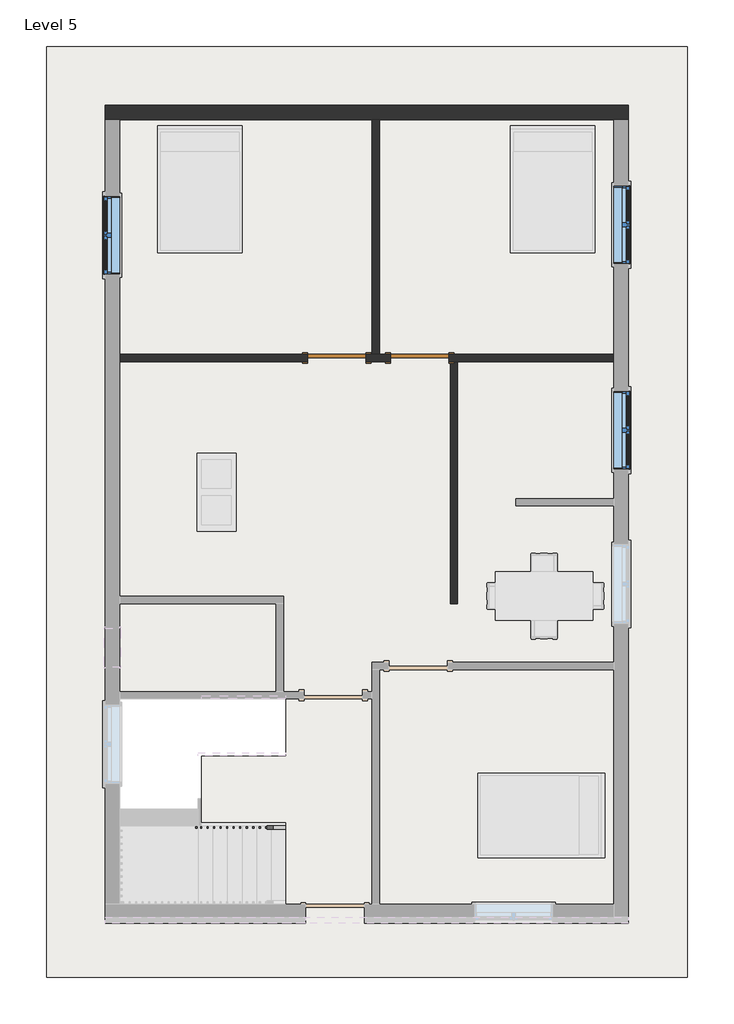
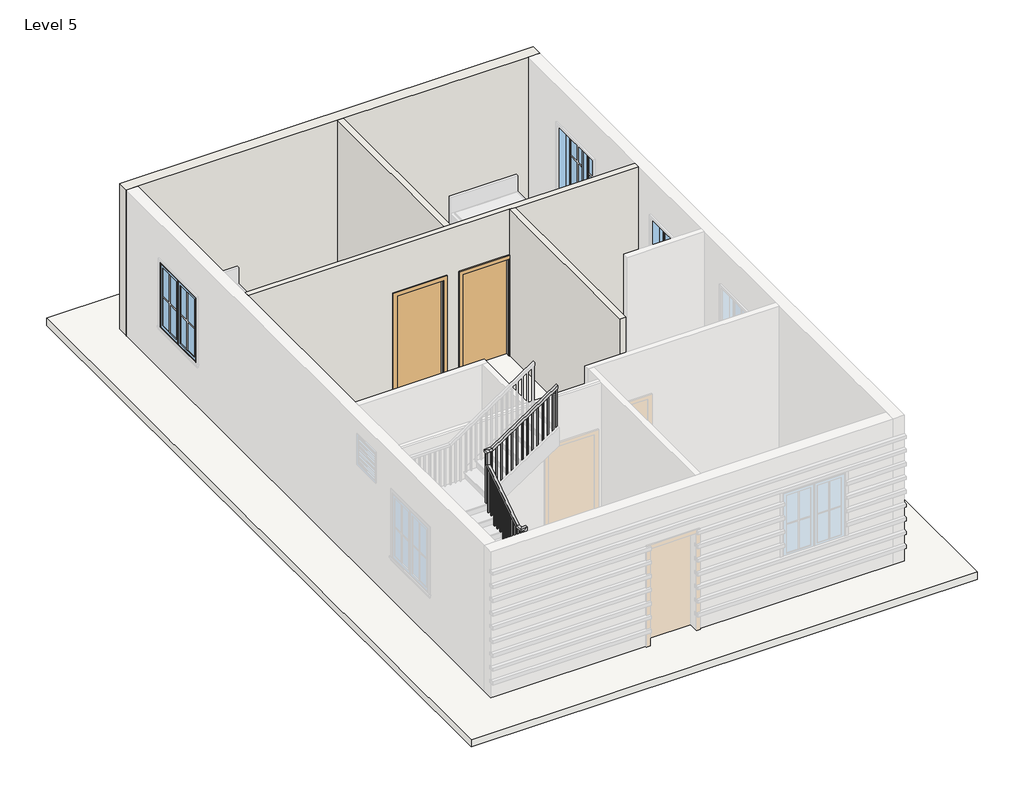
# One storey, part 2 of 3: 4 walls, 3 windows, 2 doors, 1 railing, 1 roof.
"""IFC4 building model written with IfcOpenShell, lengths in millimetres."""

from ifc_helpers import new_model, si_unit, frame, origin, place, context, project, spatial, polyline, outline, extrude, faceted_brep, transform, mapped, element, save
from components import single_flush_door_3_17d80c48, single_flush_door_3_5e62189b, window_casement_double_window_4_576b2d2c

model = new_model("IFC4")

# Units and contexts
model_context = context("Model", 3, world=origin())
ifc_project = project(units=[si_unit("LENGTHUNIT", "METRE", prefix="MILLI")], contexts=[model_context])

# Site, building, storey
site = spatial("IfcSite", under=ifc_project)
building = spatial("IfcBuilding", under=site)
storey = spatial("IfcBuildingStorey", under=building, Name="Level 5", Elevation=12649.2)

# Doors
placement = place(None, origin())
single_flush_door_3_shape = single_flush_door_3_17d80c48(model_context)
element("IfcDoor", 1, ObjectType="Single-Flush : DOOR 3'", at=placement, inside=storey, context=model_context, shape_type="MappedRepresentation", body=[
    mapped(single_flush_door_3_shape, transform((-1721.4617403, 2133.1073441, 12649.2), x_axis=(1.0, 0.0, 0.0), y_axis=(0.0, 1.0, 0.0), z_axis=(0.0, 0.0, 1.0))),
])
single_flush_door_3_2_shape = single_flush_door_3_5e62189b(model_context)
element("IfcDoor", 2, ObjectType="Single-Flush : DOOR 3'", at=placement, inside=storey, context=model_context, shape_type="MappedRepresentation", body=[
    mapped(single_flush_door_3_2_shape, transform((-426.0617403, 2133.1073441, 12649.2), x_axis=(-1.0, 0.0, 0.0), y_axis=(0.0, -1.0, 0.0), z_axis=(0.0, 0.0, 1.0))),
])

# Railing
element("IfcRailing", 3, ObjectType="Handrail - Rectangular", at=placement, inside=storey, context=model_context, shape_type="SolidModel", body=[
    faceted_brep([(-2515.2117403, -5213.8426559, 13716.0), (-2515.2117403, -5213.8426559, 13654.9459984), (-2515.2117403, -5163.0426559, 13654.9459984), (-2515.2117403, -5163.0426559, 13716.0), (-3810.6117403, -5213.8426559, 14579.6), (-3861.4117403, -5213.8426559, 14552.4126651), (-3861.4117403, -5163.0426559, 14552.4126651), (-3810.6117403, -5163.0426559, 14579.6), (-3810.6117403, -5213.8426559, 14833.6), (-3861.4117403, -5213.8426559, 14782.8), (-3861.4117403, -5163.0426559, 14782.8), (-3810.6117403, -5163.0426559, 14833.6), (-3937.6117403, -5213.8426559, 14833.6), (-3937.6117403, -5213.8426559, 14782.8), (-3886.8117403, -5163.0426559, 14782.8), (-3886.8117403, -5163.0426559, 14833.6), (-3937.6117403, -5086.8426559, 14833.6), (-3937.6117403, -5071.4616535, 14782.8), (-3886.8117403, -5071.4616535, 14782.8), (-3886.8117403, -5086.8426559, 14833.6), (-3937.6117403, -4096.2426559, 15494.0), (-3937.6117403, -4045.4426559, 15466.8126651), (-3886.8117403, -4045.4426559, 15466.8126651), (-3886.8117403, -4096.2426559, 15494.0), (-3937.6117403, -4096.2426559, 15748.0), (-3937.6117403, -4045.4426559, 15697.2), (-3886.8117403, -4045.4426559, 15697.2), (-3886.8117403, -4096.2426559, 15748.0), (-3937.6117403, -3969.2426559, 15748.0), (-3937.6117403, -3969.2426559, 15697.2), (-3886.8117403, -4020.0426559, 15697.2), (-3886.8117403, -4020.0426559, 15748.0), (-3810.6117403, -3969.2426559, 15748.0), (-3795.2307379, -3969.2426559, 15697.2), (-3795.2307379, -4020.0426559, 15697.2), (-3810.6117403, -4020.0426559, 15748.0), (-2515.2117403, -3969.2426559, 16611.6), (-2515.2117403, -4020.0426559, 16611.6), (-2515.2117403, -4020.0426559, 16550.5459984), (-2515.2117403, -3969.2426559, 16550.5459984)], [[[0, 1, 2, 3]], [[1, 0, 4, 5]], [[2, 1, 5, 6]], [[3, 2, 6, 7]], [[0, 3, 7, 4]], [[5, 4, 8, 9]], [[6, 5, 9, 10]], [[7, 6, 10, 11]], [[4, 7, 11, 8]], [[9, 8, 12, 13]], [[10, 9, 13, 14]], [[11, 10, 14, 15]], [[8, 11, 15, 12]], [[13, 12, 16, 17]], [[14, 13, 17, 18]], [[15, 14, 18, 19]], [[12, 15, 19, 16]], [[17, 16, 20, 21]], [[18, 17, 21, 22]], [[19, 18, 22, 23]], [[16, 19, 23, 20]], [[21, 20, 24, 25]], [[22, 21, 25, 26]], [[23, 22, 26, 27]], [[20, 23, 27, 24]], [[25, 24, 28, 29]], [[26, 25, 29, 30]], [[27, 26, 30, 31]], [[24, 27, 31, 28]], [[29, 28, 32, 33]], [[30, 29, 33, 34]], [[31, 30, 34, 35]], [[28, 31, 35, 32]], [[36, 37, 38, 39]], [[33, 32, 36, 39]], [[34, 33, 39, 38]], [[35, 34, 38, 37]], [[32, 35, 37, 36]]]),
    extrude(outline(polyline([(16506.0959984, -2581.8867403), (16493.3959984, -2600.9367403), (15544.8, -2600.9367403), (15544.8, -2581.8867403), (16506.0959984, -2581.8867403)])), frame((0.0, -4004.1676559, 0.0), z_axis=(0.0, 1.0, 0.0), x_axis=(0.0, 0.0, 1.0)), (0.0, 0.0, 1.0), 19.05),
    extrude(outline(polyline([(16438.3626651, -2683.4867403), (16425.6626651, -2702.5367403), (15544.8, -2702.5367403), (15544.8, -2683.4867403), (16438.3626651, -2683.4867403)])), frame((0.0, -4004.1676559, 0.0), z_axis=(0.0, 1.0, 0.0), x_axis=(0.0, 0.0, 1.0)), (0.0, 0.0, 1.0), 19.05),
    extrude(outline(polyline([(16370.6293317, -2785.0867403), (16357.9293317, -2804.1367403), (15392.4, -2804.1367403), (15392.4, -2785.0867403), (16370.6293317, -2785.0867403)])), frame((0.0, -4004.1676559, 0.0), z_axis=(0.0, 1.0, 0.0), x_axis=(0.0, 0.0, 1.0)), (0.0, 0.0, 1.0), 19.05),
    extrude(outline(polyline([(16302.8959984, -2886.6867403), (16290.1959984, -2905.7367403), (15392.4, -2905.7367403), (15392.4, -2886.6867403), (16302.8959984, -2886.6867403)])), frame((0.0, -4004.1676559, 0.0), z_axis=(0.0, 1.0, 0.0), x_axis=(0.0, 0.0, 1.0)), (0.0, 0.0, 1.0), 19.05),
    extrude(outline(polyline([(16235.1626651, -2988.2867403), (16222.4626651, -3007.3367403), (15240.0, -3007.3367403), (15240.0, -2988.2867403), (16235.1626651, -2988.2867403)])), frame((0.0, -4004.1676559, 0.0), z_axis=(0.0, 1.0, 0.0), x_axis=(0.0, 0.0, 1.0)), (0.0, 0.0, 1.0), 19.05),
    extrude(outline(polyline([(16167.4293317, -3089.8867403), (16154.7293317, -3108.9367403), (15240.0, -3108.9367403), (15240.0, -3089.8867403), (16167.4293317, -3089.8867403)])), frame((0.0, -4004.1676559, 0.0), z_axis=(0.0, 1.0, 0.0), x_axis=(0.0, 0.0, 1.0)), (0.0, 0.0, 1.0), 19.05),
    extrude(outline(polyline([(16099.6959984, -3191.4867403), (16086.9959984, -3210.5367403), (15240.0, -3210.5367403), (15240.0, -3191.4867403), (16099.6959984, -3191.4867403)])), frame((0.0, -4004.1676559, 0.0), z_axis=(0.0, 1.0, 0.0), x_axis=(0.0, 0.0, 1.0)), (0.0, 0.0, 1.0), 19.05),
    extrude(outline(polyline([(16031.9626651, -3293.0867403), (16019.2626651, -3312.1367403), (15087.6, -3312.1367403), (15087.6, -3293.0867403), (16031.9626651, -3293.0867403)])), frame((0.0, -4004.1676559, 0.0), z_axis=(0.0, 1.0, 0.0), x_axis=(0.0, 0.0, 1.0)), (0.0, 0.0, 1.0), 19.05),
    extrude(outline(polyline([(15964.2293317, -3394.6867403), (15951.5293317, -3413.7367403), (15087.6, -3413.7367403), (15087.6, -3394.6867403), (15964.2293317, -3394.6867403)])), frame((0.0, -4004.1676559, 0.0), z_axis=(0.0, 1.0, 0.0), x_axis=(0.0, 0.0, 1.0)), (0.0, 0.0, 1.0), 19.05),
    extrude(outline(polyline([(15896.4959984, -3496.2867403), (15883.7959984, -3515.3367403), (14935.2, -3515.3367403), (14935.2, -3496.2867403), (15896.4959984, -3496.2867403)])), frame((0.0, -4004.1676559, 0.0), z_axis=(0.0, 1.0, 0.0), x_axis=(0.0, 0.0, 1.0)), (0.0, 0.0, 1.0), 19.05),
    extrude(outline(polyline([(15828.7626651, -3597.8867403), (15816.0626651, -3616.9367403), (14935.2, -3616.9367403), (14935.2, -3597.8867403), (15828.7626651, -3597.8867403)])), frame((0.0, -4004.1676559, 0.0), z_axis=(0.0, 1.0, 0.0), x_axis=(0.0, 0.0, 1.0)), (0.0, 0.0, 1.0), 19.05),
    extrude(outline(polyline([(15761.0293317, -3699.4867403), (15748.3293317, -3718.5367403), (14782.8, -3718.5367403), (14782.8, -3699.4867403), (15761.0293317, -3699.4867403)])), frame((0.0, -4004.1676559, 0.0), z_axis=(0.0, 1.0, 0.0), x_axis=(0.0, 0.0, 1.0)), (0.0, 0.0, 1.0), 19.05),
    extrude(outline(polyline([(15693.2959984, -3801.0867403), (15680.5959984, -3820.1367403), (14782.8, -3820.1367403), (14782.8, -3801.0867403), (15693.2959984, -3801.0867403)])), frame((0.0, -4004.1676559, 0.0), z_axis=(0.0, 1.0, 0.0), x_axis=(0.0, 0.0, 1.0)), (0.0, 0.0, 1.0), 19.05),
    extrude(outline(polyline([(-3902.6867403, -4080.3676559), (-3921.7367403, -4080.3676559), (-3921.7367403, -4061.3176559), (-3902.6867403, -4061.3176559), (-3902.6867403, -4080.3676559)])), frame((0.0, 0.0, 14478.0), z_axis=(0.0, 0.0, 1.0), x_axis=(1.0, 0.0, 0.0)), (0.0, 0.0, 1.0), 1219.2),
    extrude(outline(polyline([(-4181.9676559, 15375.7959984), (-4162.9176559, 15388.4959984), (-4162.9176559, 14478.0), (-4181.9676559, 14478.0), (-4181.9676559, 15375.7959984)])), frame((-3921.7367403, 0.0, 0.0), z_axis=(1.0, 0.0, 0.0), x_axis=(0.0, 1.0, 0.0)), (0.0, 0.0, 1.0), 19.05),
    extrude(outline(polyline([(-4283.5676559, 15308.0626651), (-4264.5176559, 15320.7626651), (-4264.5176559, 14325.6), (-4283.5676559, 14325.6), (-4283.5676559, 15308.0626651)])), frame((-3921.7367403, 0.0, 0.0), z_axis=(1.0, 0.0, 0.0), x_axis=(0.0, 1.0, 0.0)), (0.0, 0.0, 1.0), 19.05),
    extrude(outline(polyline([(-4385.1676559, 15240.3293317), (-4366.1176559, 15253.0293317), (-4366.1176559, 14325.6), (-4385.1676559, 14325.6), (-4385.1676559, 15240.3293317)])), frame((-3921.7367403, 0.0, 0.0), z_axis=(1.0, 0.0, 0.0), x_axis=(0.0, 1.0, 0.0)), (0.0, 0.0, 1.0), 19.05),
    extrude(outline(polyline([(-4486.7676559, 15172.5959984), (-4467.7176559, 15185.2959984), (-4467.7176559, 14325.6), (-4486.7676559, 14325.6), (-4486.7676559, 15172.5959984)])), frame((-3921.7367403, 0.0, 0.0), z_axis=(1.0, 0.0, 0.0), x_axis=(0.0, 1.0, 0.0)), (0.0, 0.0, 1.0), 19.05),
    extrude(outline(polyline([(-4588.3676559, 15104.8626651), (-4569.3176559, 15117.5626651), (-4569.3176559, 14173.2), (-4588.3676559, 14173.2), (-4588.3676559, 15104.8626651)])), frame((-3921.7367403, 0.0, 0.0), z_axis=(1.0, 0.0, 0.0), x_axis=(0.0, 1.0, 0.0)), (0.0, 0.0, 1.0), 19.05),
    extrude(outline(polyline([(-4689.9676559, 15037.1293317), (-4670.9176559, 15049.8293317), (-4670.9176559, 14173.2), (-4689.9676559, 14173.2), (-4689.9676559, 15037.1293317)])), frame((-3921.7367403, 0.0, 0.0), z_axis=(1.0, 0.0, 0.0), x_axis=(0.0, 1.0, 0.0)), (0.0, 0.0, 1.0), 19.05),
    extrude(outline(polyline([(-4791.5676559, 14969.3959984), (-4772.5176559, 14982.0959984), (-4772.5176559, 14020.8), (-4791.5676559, 14020.8), (-4791.5676559, 14969.3959984)])), frame((-3921.7367403, 0.0, 0.0), z_axis=(1.0, 0.0, 0.0), x_axis=(0.0, 1.0, 0.0)), (0.0, 0.0, 1.0), 19.05),
    extrude(outline(polyline([(-4893.1676559, 14901.6626651), (-4874.1176559, 14914.3626651), (-4874.1176559, 14020.8), (-4893.1676559, 14020.8), (-4893.1676559, 14901.6626651)])), frame((-3921.7367403, 0.0, 0.0), z_axis=(1.0, 0.0, 0.0), x_axis=(0.0, 1.0, 0.0)), (0.0, 0.0, 1.0), 19.05),
    extrude(outline(polyline([(-4994.7676559, 14833.9293317), (-4975.7176559, 14846.6293317), (-4975.7176559, 13868.4), (-4994.7676559, 13868.4), (-4994.7676559, 14833.9293317)])), frame((-3921.7367403, 0.0, 0.0), z_axis=(1.0, 0.0, 0.0), x_axis=(0.0, 1.0, 0.0)), (0.0, 0.0, 1.0), 19.05),
    extrude(outline(polyline([(-5096.3676559, 14766.1959984), (-5077.3176559, 14778.8959984), (-5077.3176559, 13868.4), (-5096.3676559, 13868.4), (-5096.3676559, 14766.1959984)])), frame((-3921.7367403, 0.0, 0.0), z_axis=(1.0, 0.0, 0.0), x_axis=(0.0, 1.0, 0.0)), (0.0, 0.0, 1.0), 19.05),
    extrude(outline(polyline([(-3826.4867403, -5178.9176559), (-3826.4867403, -5197.9676559), (-3845.5367403, -5197.9676559), (-3845.5367403, -5178.9176559), (-3826.4867403, -5178.9176559)])), frame((0.0, 0.0, 13563.6), z_axis=(0.0, 0.0, 1.0), x_axis=(1.0, 0.0, 0.0)), (0.0, 0.0, 1.0), 1219.2),
    extrude(outline(polyline([(14461.3959984, -3724.8867403), (14474.0959984, -3743.9367403), (13563.6, -3743.9367403), (13563.6, -3724.8867403), (14461.3959984, -3724.8867403)])), frame((0.0, -5197.9676559, 0.0), z_axis=(0.0, 1.0, 0.0), x_axis=(0.0, 0.0, 1.0)), (0.0, 0.0, 1.0), 19.05),
    extrude(outline(polyline([(14393.6626651, -3623.2867403), (14406.3626651, -3642.3367403), (13411.2, -3642.3367403), (13411.2, -3623.2867403), (14393.6626651, -3623.2867403)])), frame((0.0, -5197.9676559, 0.0), z_axis=(0.0, 1.0, 0.0), x_axis=(0.0, 0.0, 1.0)), (0.0, 0.0, 1.0), 19.05),
    extrude(outline(polyline([(14325.9293317, -3521.6867403), (14338.6293317, -3540.7367403), (13411.2, -3540.7367403), (13411.2, -3521.6867403), (14325.9293317, -3521.6867403)])), frame((0.0, -5197.9676559, 0.0), z_axis=(0.0, 1.0, 0.0), x_axis=(0.0, 0.0, 1.0)), (0.0, 0.0, 1.0), 19.05),
    extrude(outline(polyline([(14258.1959984, -3420.0867403), (14270.8959984, -3439.1367403), (13411.2, -3439.1367403), (13411.2, -3420.0867403), (14258.1959984, -3420.0867403)])), frame((0.0, -5197.9676559, 0.0), z_axis=(0.0, 1.0, 0.0), x_axis=(0.0, 0.0, 1.0)), (0.0, 0.0, 1.0), 19.05),
    extrude(outline(polyline([(14190.4626651, -3318.4867403), (14203.1626651, -3337.5367403), (13258.8, -3337.5367403), (13258.8, -3318.4867403), (14190.4626651, -3318.4867403)])), frame((0.0, -5197.9676559, 0.0), z_axis=(0.0, 1.0, 0.0), x_axis=(0.0, 0.0, 1.0)), (0.0, 0.0, 1.0), 19.05),
    extrude(outline(polyline([(14122.7293317, -3216.8867403), (14135.4293317, -3235.9367403), (13258.8, -3235.9367403), (13258.8, -3216.8867403), (14122.7293317, -3216.8867403)])), frame((0.0, -5197.9676559, 0.0), z_axis=(0.0, 1.0, 0.0), x_axis=(0.0, 0.0, 1.0)), (0.0, 0.0, 1.0), 19.05),
    extrude(outline(polyline([(14054.9959984, -3115.2867403), (14067.6959984, -3134.3367403), (13106.4, -3134.3367403), (13106.4, -3115.2867403), (14054.9959984, -3115.2867403)])), frame((0.0, -5197.9676559, 0.0), z_axis=(0.0, 1.0, 0.0), x_axis=(0.0, 0.0, 1.0)), (0.0, 0.0, 1.0), 19.05),
    extrude(outline(polyline([(13987.2626651, -3013.6867403), (13999.9626651, -3032.7367403), (13106.4, -3032.7367403), (13106.4, -3013.6867403), (13987.2626651, -3013.6867403)])), frame((0.0, -5197.9676559, 0.0), z_axis=(0.0, 1.0, 0.0), x_axis=(0.0, 0.0, 1.0)), (0.0, 0.0, 1.0), 19.05),
    extrude(outline(polyline([(13919.5293317, -2912.0867403), (13932.2293317, -2931.1367403), (12954.0, -2931.1367403), (12954.0, -2912.0867403), (13919.5293317, -2912.0867403)])), frame((0.0, -5197.9676559, 0.0), z_axis=(0.0, 1.0, 0.0), x_axis=(0.0, 0.0, 1.0)), (0.0, 0.0, 1.0), 19.05),
    extrude(outline(polyline([(13851.7959984, -2810.4867403), (13864.4959984, -2829.5367403), (12954.0, -2829.5367403), (12954.0, -2810.4867403), (13851.7959984, -2810.4867403)])), frame((0.0, -5197.9676559, 0.0), z_axis=(0.0, 1.0, 0.0), x_axis=(0.0, 0.0, 1.0)), (0.0, 0.0, 1.0), 19.05),
    extrude(outline(polyline([(13784.0626651, -2708.8867403), (13796.7626651, -2727.9367403), (12801.6, -2727.9367403), (12801.6, -2708.8867403), (13784.0626651, -2708.8867403)])), frame((0.0, -5197.9676559, 0.0), z_axis=(0.0, 1.0, 0.0), x_axis=(0.0, 0.0, 1.0)), (0.0, 0.0, 1.0), 19.05),
    extrude(outline(polyline([(13716.3293317, -2607.2867403), (13729.0293317, -2626.3367403), (12801.6, -2626.3367403), (12801.6, -2607.2867403), (13716.3293317, -2607.2867403)])), frame((0.0, -5197.9676559, 0.0), z_axis=(0.0, 1.0, 0.0), x_axis=(0.0, 0.0, 1.0)), (0.0, 0.0, 1.0), 19.05),
    extrude(outline(polyline([(-3902.6867403, -4004.1676559), (-3921.7367403, -4004.1676559), (-3921.7367403, -3985.1176559), (-3902.6867403, -3985.1176559), (-3902.6867403, -4004.1676559)])), frame((0.0, 0.0, 14630.4), z_axis=(0.0, 0.0, 1.0), x_axis=(1.0, 0.0, 0.0)), (0.0, 0.0, 1.0), 1066.8),
    extrude(outline(polyline([(-3902.6867403, -5178.9176559), (-3902.6867403, -5197.9676559), (-3921.7367403, -5197.9676559), (-3921.7367403, -5178.9176559), (-3902.6867403, -5178.9176559)])), frame((0.0, 0.0, 13716.0), z_axis=(0.0, 0.0, 1.0), x_axis=(1.0, 0.0, 0.0)), (0.0, 0.0, 1.0), 1066.8),
    extrude(outline(polyline([(16550.5459984, -2515.2117403), (16537.8459984, -2534.2617403), (15544.8, -2534.2617403), (15544.8, -2515.2117403), (16550.5459984, -2515.2117403)])), frame((0.0, -4004.1676559, 0.0), z_axis=(0.0, 1.0, 0.0), x_axis=(0.0, 0.0, 1.0)), (0.0, 0.0, 1.0), 19.05),
    extrude(outline(polyline([(13654.9459984, -2515.2117403), (13667.6459984, -2534.2617403), (12801.6, -2534.2617403), (12801.6, -2515.2117403), (13654.9459984, -2515.2117403)])), frame((0.0, -5197.9676559, 0.0), z_axis=(0.0, 1.0, 0.0), x_axis=(0.0, 0.0, 1.0)), (0.0, 0.0, 1.0), 19.05),
])

# Roof
element("IfcRoof", 4, ObjectType="ROOF 6\"", at=placement, inside=storey, context=model_context, shape_type="SweptSolid", body=[
    extrude(outline(polyline([(-6249.0117403, -7525.2426559), (-6249.0117403, 6990.8573441), (3745.8882597, 6990.8573441), (3745.8882597, -7525.2426559), (-6249.0117403, -7525.2426559)]), holes=[polyline([(-5156.8117403, -3131.0426559), (-5156.8117403, -6433.0426559), (-2515.2117403, -6433.0426559), (-2515.2117403, -5112.2426559), (-3836.0117403, -5112.2426559), (-3836.0117403, -4070.8426559), (-2515.2117403, -4070.8426559), (-2515.2117403, -3131.0426559), (-5156.8117403, -3131.0426559)])]), frame((0.0, 0.0, 12496.8), z_axis=(0.0, 0.0, 1.0), x_axis=(1.0, 0.0, 0.0)), (0.0, 0.0, 1.0), 152.4),
])

# Walls
element("IfcWall", 5, ObjectType="ALL 4.5\"", at=placement, inside=storey, context=model_context, shape_type="Brep", body=[
    faceted_brep([(-1264.2617403, 2075.9573441, 12649.2), (-883.2617403, 2075.9573441, 12649.2), (-883.2617403, 2075.9573441, 14681.2), (31.1382597, 2075.9573441, 14681.2), (31.1382597, 2075.9573441, 12649.2), (50.1882597, 2075.9573441, 12649.2), (164.4882597, 2075.9573441, 12649.2), (2602.8882597, 2075.9573441, 12649.2), (2602.8882597, 2075.9573441, 15697.2), (164.4882597, 2075.9573441, 15697.2), (50.1882597, 2075.9573441, 15697.2), (-5106.0117403, 2075.9573441, 15697.2), (-5106.0117403, 2075.9573441, 12649.2), (-2178.6617403, 2075.9573441, 12649.2), (-2178.6617403, 2075.9573441, 14681.2), (-1264.2617403, 2075.9573441, 14681.2), (-883.2617403, 2190.2573441, 14681.2), (-883.2617403, 2190.2573441, 12649.2), (-1054.7117403, 2190.2573441, 12649.2), (-1169.0117403, 2190.2573441, 12649.2), (-1264.2617403, 2190.2573441, 12649.2), (-1264.2617403, 2190.2573441, 14681.2), (-2178.6617403, 2190.2573441, 14681.2), (-2178.6617403, 2190.2573441, 12649.2), (-5106.0117403, 2190.2573441, 12649.2), (-5106.0117403, 2190.2573441, 15697.2), (-1169.0117403, 2190.2573441, 15697.2), (-1054.7117403, 2190.2573441, 15697.2), (2602.8882597, 2190.2573441, 15697.2), (2602.8882597, 2190.2573441, 12649.2), (31.1382597, 2190.2573441, 12649.2), (31.1382597, 2190.2573441, 14681.2)], [[[0, 1, 2, 3, 4, 5, 6, 7, 8, 9, 10, 11, 12, 13, 14, 15]], [[16, 17, 18, 19, 20, 21, 22, 23, 24, 25, 26, 27, 28, 29, 30, 31]], [[13, 12, 24, 23]], [[30, 29, 7, 6, 5, 4]], [[20, 19, 18, 17, 1, 0]], [[8, 7, 29, 28]], [[12, 11, 25, 24]], [[21, 20, 0, 15]], [[22, 21, 15, 14]], [[23, 22, 14, 13]], [[2, 1, 17, 16]], [[3, 2, 16, 31]], [[4, 3, 31, 30]], [[11, 10, 9, 8, 28, 27, 26, 25]]]),
])
element("IfcWall", 6, ObjectType="ALL 4.5\"", at=placement, inside=storey, context=model_context, shape_type="SweptSolid", body=[
    extrude(outline(polyline([(50.1882597, -1695.9426559), (50.1882597, 2075.9573441), (164.4882597, 2075.9573441), (164.4882597, -1695.9426559), (50.1882597, -1695.9426559)])), frame((0.0, 0.0, 12649.2), z_axis=(0.0, 0.0, 1.0), x_axis=(1.0, 0.0, 0.0)), (0.0, 0.0, 1.0), 3048.0),
])
element("IfcWall", 7, ObjectType="ALL 4.5\"", at=placement, inside=storey, context=model_context, shape_type="SweptSolid", body=[
    extrude(outline(polyline([(-1169.0117403, 2190.2573441), (-1169.0117403, 5847.8573441), (-1054.7117403, 5847.8573441), (-1054.7117403, 2190.2573441), (-1169.0117403, 2190.2573441)])), frame((0.0, 0.0, 12649.2), z_axis=(0.0, 0.0, 1.0), x_axis=(1.0, 0.0, 0.0)), (0.0, 0.0, 1.0), 3048.0),
])
element("IfcWall", 8, ObjectType="WALL 9\"", at=placement, inside=storey, context=model_context, shape_type="Brep", body=[
    faceted_brep([(-5334.6117403, 5847.8573441, 12649.2), (-5106.0117403, 5847.8573441, 12649.2), (-1169.0117403, 5847.8573441, 12649.2), (-1054.7117403, 5847.8573441, 12649.2), (2602.8882597, 5847.8573441, 12649.2), (2831.4882597, 5847.8573441, 12649.2), (2831.4882597, 5847.8573441, 15697.2), (2602.8882597, 5847.8573441, 15697.2), (-1054.7117403, 5847.8573441, 15697.2), (-1169.0117403, 5847.8573441, 15697.2), (-5106.0117403, 5847.8573441, 15697.2), (-5334.6117403, 5847.8573441, 15697.2), (-5334.6117403, 6076.4573441, 12649.2), (-5334.6117403, 6076.4573441, 15697.2), (2831.4882597, 6076.4573441, 15697.2), (2831.4882597, 6076.4573441, 12649.2)], [[[0, 1, 2, 3, 4, 5, 6, 7, 8, 9, 10, 11]], [[12, 13, 14, 15]], [[5, 4, 3, 2, 1, 0, 12, 15]], [[6, 5, 15, 14]], [[0, 11, 13, 12]], [[11, 10, 9, 8, 7, 6, 14, 13]]]),
])

# Windows
window_casement_double_window_4_shape = window_casement_double_window_4_576b2d2c(model_context)
element("IfcWindow", 9, ObjectType="Window-Casement-Double : WINDOW 4'", at=placement, inside=storey, context=model_context, shape_type="MappedRepresentation", body=[
    mapped(window_casement_double_window_4_shape, transform((-5220.3117403, 4047.6323441, 12649.2), x_axis=(0.0, 1.0, 0.0), y_axis=(-1.0, 0.0, 0.0), z_axis=(0.0, 0.0, 1.0))),
])
element("IfcWindow", 10, ObjectType="Window-Casement-Double : WINDOW 4'", at=placement, inside=storey, context=model_context, shape_type="MappedRepresentation", body=[
    mapped(window_casement_double_window_4_shape, transform((2717.1882597, 4209.5573441, 12649.2), x_axis=(0.0, -1.0, 0.0), y_axis=(1.0, 0.0, 0.0), z_axis=(0.0, 0.0, 1.0))),
])
element("IfcWindow", 11, ObjectType="Window-Casement-Double : WINDOW 4'", at=placement, inside=storey, context=model_context, shape_type="MappedRepresentation", body=[
    mapped(window_casement_double_window_4_shape, transform((2717.1882597, 1009.1573441, 12649.2), x_axis=(0.0, -1.0, 0.0), y_axis=(1.0, 0.0, 0.0), z_axis=(0.0, 0.0, 1.0))),
])

save(model, "model.ifc")

# Revit data of these elements
# Type "Single-Flush : DOOR 3'"
#   Type Mark = "8"
#   Construction Type Id = "MDOOR"
#   Assembly Code = "C1020"
#   Analytic Construction = "Metal"
#   Thickness = 0' - 2"
#   Heat Transfer Coefficient (U) = 0.651978 BTU/(h·ft²·°F)
#   Height = 6' - 8"
#   Trim Projection Ext = 0' - 1"
#   Trim Projection Int = 0' - 1"
#   Trim Width = 0' - 3"
#   Width = 3' - 0"
#   Define Thermal Properties by = 1
#   Door Material = Door - Panel
#   Frame Material = Door - Frame
#   Visual Light Transmittance = 0
#   Solar Heat Gain Coefficient = 0
#   Function = (empty or 0)
#   Wall Closure = (empty or 0)
# Type "Handrail - Rectangular"
#   Assembly Code = "C2010400"
#   built-in parameter 1008612 = 0.0416667 (stored number, unit not read)
#   built-in parameter 1008611 = 0.0416667 (stored number, unit not read)
#   built-in parameter 1008609 = 0.333333 (stored number, unit not read)
#   built-in parameter 1008604 = 0.166667 (stored number, unit not read)
#   built-in parameter 1008603 = 0.166667 (stored number, unit not read)
#   Railing Height = 3' - 0"
#   built-in parameter 1008630 = 2
#   built-in parameter 1008610 = 2
#   built-in parameter 1008618 = Baluster - Square : 3/4"
# Type "ROOF 6\""
#   Assembly Code = "B1020"
#   Layers, outside or top first: 0' - 6" no material (function 1)
# Type "ALL 4.5\""
#   Assembly Code = "B2010"
#   Layers, outside or top first: 0' - 4 1/2" no material (function 1)
# Type "WALL 9\""
#   Assembly Code = "B2010"
#   Layers, outside or top first: 0' - 9" "Carpet (1)" (function 1)
# Type "Window-Casement-Double : WINDOW 4'"
#   Type Mark = "18"
#   Fire Rating = "0.5h"
#   Assembly Code = "B2020100"
#   Analytic Construction = "Double glazing - domestic"
#   Frame Extension [instance default] = 0' - 0 1/4"
#   Window Inset [instance default] = 0' - 0"
#   Wall Thickness [instance default] = 0' - 6"
#   Interior Wall Closure [instance default] = 0' - 2 1/4"
#   Half Width = 2' - 0"
#   Visual Light Transmittance = 0.81
#   Thermal Resistance (R) = 1.8146 (h·ft²·°F)/BTU
#   Solar Heat Gain Coefficient = 0.76
#   Rough Width = 4' - 0 1/2"
#   Rough Height = 4' - 5 1/2"
#   Height = 4' - 5"
#   Heat Transfer Coefficient (U) = 0.5511 BTU/(h·ft²·°F)
#   Exterior Wall Closure [instance default] = 0' - 1 1/4"
#   Extension Jamb [instance default] = 0' - 2 1/4"
#   Default Sill Height = 3' - 0"
#   Width = 4' - 0"
#   Muntin Visibility = yes
#   Interior Trim Visibility [instance default] = yes
#   Exterior Trim Visibility [instance default] = yes
#   Extension Jamb Visibility [instance default] = yes
#   Interior Trim Material = Wood - Stained
#   Muntin Pattern = Muntin Pattern_2x2 : Muntin Pattern_2x2
#   Interior Trim = Trim-Window-Interior-Flat : Picture Frame
#   Interior Frame Material = Wood - Stained
#   Glass Panel Material = Glass
#   Exterior Trim Material = Clad - White
#   Exterior Trim = Trim-Window-Exterior-Flat : with Sill
#   Exterior Frame Material = Clad - White
#   Wall Closure = (empty or 0)
# Elements 1, 2 (IfcDoor, "Single-Flush : DOOR 3'")
#   Phase Created = New Construction
#   Materials on its faces: "Door - Frame", "Door - Panel"
# Element 3 (IfcRailing, "Handrail - Rectangular")
#   Phase Created = New Construction
#   Materials on its faces: "Clad - White"
# Element 4 (IfcRoof, "ROOF 6\"")
#   built-in parameter 1001705 = 41.5 (stored number, unit not read)
#   built-in parameter 1001701 = -0.5 (stored number, unit not read)
#   built-in parameter 1001710 = 33615
#   Phase Created = New Construction
#   Materials on its faces: "Clad - White", "Default Roof", "Softwood, Lumber"
# Elements 5, 6, 7 (IfcWall, "ALL 4.5\"")
#   Top Offset = 0' - 0"
#   Base Offset = 0' - 0"
#   Unconnected Height = 10' - 0"
#   wall height = 10' - 0"
#   Phase Created = New Construction
#   Base Constraint = Level 5
#   Materials on its faces: "Default Wall"
# Element 8 (IfcWall, "WALL 9\"")
#   Top Offset = 0' - 0"
#   Base Offset = 0' - 0"
#   Unconnected Height = 10' - 0"
#   wall height = 10' - 0"
#   Phase Created = New Construction
#   Base Constraint = Level 5
#   Materials on its faces: "Carpet (1)", "Wood - Stained"
# Element 9 (IfcWindow, "Window-Casement-Double : WINDOW 4'")
#   Mark = "30"
#   Window Inset = 0' - 0"
#   Interior Wall Closure = 0' - 2 1/4"
#   Frame Extension = 0' - 0 1/4"
#   Exterior Wall Closure = 0' - 1 1/4"
#   Interior Trim Visibility = yes
#   Exterior Trim Visibility = yes
#   Phase Created = New Construction
#   Materials on its faces: "Wood - Stained", "Glass", "Clad - White"
# Element 10 (IfcWindow, "Window-Casement-Double : WINDOW 4'")
#   Mark = "31"
#   Window Inset = 0' - 0"
#   Interior Wall Closure = 0' - 2 1/4"
#   Frame Extension = 0' - 0 1/4"
#   Exterior Wall Closure = 0' - 1 1/4"
#   Interior Trim Visibility = yes
#   Exterior Trim Visibility = yes
#   Phase Created = New Construction
#   Materials on its faces: "Wood - Stained", "Glass", "Clad - White"
# Element 11 (IfcWindow, "Window-Casement-Double : WINDOW 4'")
#   Mark = "32"
#   Window Inset = 0' - 0"
#   Interior Wall Closure = 0' - 2 1/4"
#   Frame Extension = 0' - 0 1/4"
#   Exterior Wall Closure = 0' - 1 1/4"
#   Interior Trim Visibility = yes
#   Exterior Trim Visibility = yes
#   Phase Created = New Construction
#   Materials on its faces: "Wood - Stained", "Glass", "Clad - White"
# Materials
#   "Door - Panel": class "Wood", colour RGB 210 159 95, transparency 0, Cost = 0
#   "Door - Frame": colour RGB 118 70 51, transparency 0, Cost = 0
#   "Carpet (1)": class "Carpet", colour RGB 124 80 67, transparency 0, Description = "Interior finish", Cost = 0
#   "Wood - Stained": class "Wood", colour RGB 224 178 126, transparency 0, Cost = 0
#   "Glass": class "Glass", colour RGB 0 128 192, transparency 0.75, Description = "Soda Lime Glass", Cost = 0
#   "Clad - White": class "Wood", colour RGB 242 242 238, transparency 0, Cost = 0
#   "Default Roof": colour RGB 88 101 114, transparency 0, Cost = 0
#   "Softwood, Lumber": class "Wood", colour RGB 223 192 134, transparency 0, Description = "Pinus Echinata", Cost = 0
#   "Default Wall": colour RGB 128 128 128, transparency 0, Cost = 0
